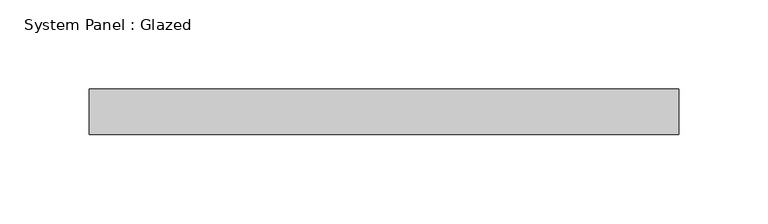
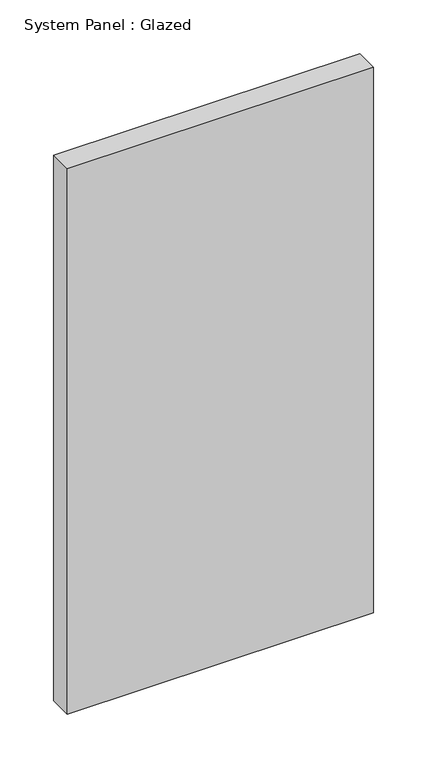
"""IFC4 building model written with IfcOpenShell, lengths in millimetres: plate geometry, System Panel : Glazed."""

from ifc_helpers import new_model, si_unit, origin, origin_with_axes, place, context, project, spatial, polyline, outline, extrude, source, transform, mapped, element, save


def system_panel_glazed_8616aaf2(model_context):
    return source(origin(), model_context, "Body", "SweptSolid", [
        extrude(outline(polyline([(165.1, 19.05), (-165.1, 19.05), (-165.1, 44.45), (165.1, 44.45), (165.1, 19.05)])), origin_with_axes(), (0.0, 0.0, 1.0), 621.3022733),
    ])


if __name__ == "__main__":
    model = new_model("IFC4")
    model_context = context("Model", 3, world=origin())
    ifc_project = project(units=[si_unit("LENGTHUNIT", "METRE", prefix="MILLI")], contexts=[model_context])
    site = spatial("IfcSite", under=ifc_project)
    building = spatial("IfcBuilding", under=site)
    placement = place(None, origin())
    system_panel_glazed_shape = system_panel_glazed_8616aaf2(model_context)
    element("IfcPlate", 1, ObjectType="System Panel : Glazed", at=placement, inside=building, context=model_context, shape_type="MappedRepresentation", body=[
        mapped(system_panel_glazed_shape, transform((0.0, 0.0, 0.0), x_axis=(1.0, 0.0, 0.0), y_axis=(0.0, 1.0, 0.0), z_axis=(0.0, 0.0, 1.0))),
    ])
    save(model, "model.ifc")

# Revit data of these elements
# Type "System Panel : Glazed"
#   Construction Type Id = "GSP4R"
#   Analytic Construction = "1/8 in Pilkington single glazing"
#   Visual Light Transmittance = 0.9
#   Solar Heat Gain Coefficient = 0.86
#   Heat Transfer Coefficient (U) = 1.18115 BTU/(h·ft²·°F)
#   Define Thermal Properties by = 1
# Element 1 (IfcPlate, "System Panel : Glazed")
#   Materials on its faces: "Glass"
# Materials
#   "Glass": class "Glass", colour RGB 0 128 192, transparency 0.75, Description = "Soda Lime Glass", Cost = 0
